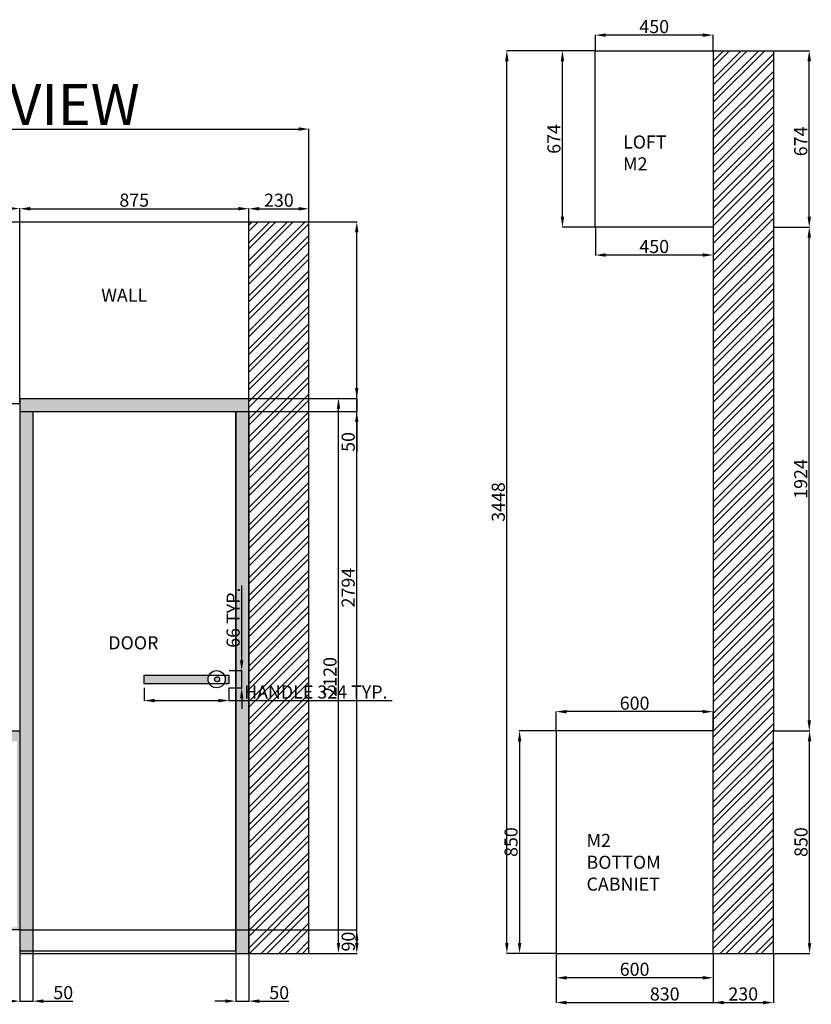
# Model space of a CAD drawing. Units: millimetres. Extents: x 144895 to 155057, y -2833 to 1092.
# Tile 4 of 4: x 152033 to 155057, y -2833 to 929. Entities that reach past the tile are written whole.
import ezdxf

# ---------------------------------------------------------------- set-up
doc = ezdxf.new("R2010")
doc.units = ezdxf.units.MM
for name, color, linetype, lineweight in [('A-ANNO-DIMS', 2, 'Continuous', 18), ('A-ANNO-TEXT', 7, 'Continuous', 18), ('A-DOOR', 4, 'Continuous', 25), ('A-ELEV', 7, 'Continuous', 25), ('A-ELEV-PATT', 252, 'Continuous', 13), ('A-WALL-PATT', 8, 'Continuous', 13)]:
    doc.layers.add(name, color=color, linetype=linetype, lineweight=lineweight)
doc.styles.get("Standard").update_dxf_attribs({"font": 'arial.ttf'})
doc.dimstyles.new('ISO-25', dxfattribs={"dimtxt": 50, "dimasz": 40, "dimexe": 1.25, "dimexo": 0.625, "dimtad": 1, "dimtxsty": 'Standard', "dimcen": 2.5, "dimadec": 0, "dimazin": 0, "dimtfac": 1, "dimtmove": 0, "dimatfit": 3, "dimfxl": 1, "dimarcsym": 0})

# ---------------------------------------------------------------- blocks, each defined once
blk = doc.blocks.new('*D1')
at = {"layer": 'A-ANNO-DIMS', "color": 0, "lineweight": -2, "transparency": 16777216}
for p, q in [((154232, 810.7), (154232, 870.9)), ((154642, 869.6), (154272, 869.6)), ((154682, 810.7), (154682, 870.9))]:
    blk.add_line(p, q, dxfattribs=at)
at = {"layer": 'A-ANNO-DIMS', "color": 0, "transparency": 16777216}
for points in [[(154272, 876.3), (154272, 863), (154232, 869.6)], [(154642, 876.3), (154642, 863), (154682, 869.6)]]:
    blk.add_solid(points, dxfattribs=at)
at = {"layer": 'Defpoints', "color": 0, "transparency": 16777216}
for p in [(154232, 869.6), (154232, 810.1), (154682, 810.1)]:
    blk.add_point(p, dxfattribs=at)
at = {"layer": 'A-ANNO-DIMS', "color": 0, "transparency": 16777216, "insert": (154457, 895.8), "char_height": 50, "attachment_point": 5}
blk.add_mtext('450', dxfattribs=at)
blk = doc.blocks.new('*D2')
at = {"layer": 'A-ANNO-DIMS', "color": 0, "lineweight": -2, "transparency": 16777216}
for p, q in [((154912.6, 810.1), (155050.3, 810.1)), ((155049, 176.1), (155049, 770.1)), ((154912.6, 136.1), (155050.3, 136.1))]:
    blk.add_line(p, q, dxfattribs=at)
at = {"layer": 'A-ANNO-DIMS', "color": 0, "transparency": 16777216}
for points in [[(155042.4, 770.1), (155055.7, 770.1), (155049, 810.1)], [(155042.4, 176.1), (155055.7, 176.1), (155049, 136.1)]]:
    blk.add_solid(points, dxfattribs=at)
at = {"layer": 'Defpoints', "color": 0, "transparency": 16777216}
for p in [(154912, 810.1), (155049, 810.1), (154912, 136.1)]:
    blk.add_point(p, dxfattribs=at)
at = {"layer": 'A-ANNO-DIMS', "color": 0, "transparency": 16777216, "insert": (155022.9, 463.7), "char_height": 50, "attachment_point": 5, "rotation": 90}
blk.add_mtext('674', dxfattribs=at)
blk = doc.blocks.new('*D3')
at = {"layer": 'A-ANNO-DIMS', "color": 0, "lineweight": -2, "transparency": 16777216}
for p, q in [((154082, -2638.5), (154082, -2732.6)), ((154682, -2638.5), (154682, -2732.6)), ((154642, -2731.3), (154122, -2731.3))]:
    blk.add_line(p, q, dxfattribs=at)
at = {"layer": 'A-ANNO-DIMS', "color": 0, "transparency": 16777216}
for points in [[(154122, -2724.7), (154122, -2738), (154082, -2731.3)], [(154642, -2724.7), (154642, -2738), (154682, -2731.3)]]:
    blk.add_solid(points, dxfattribs=at)
at = {"layer": 'Defpoints', "color": 0, "transparency": 16777216}
for p in [(154082, -2637.9), (154682, -2637.9), (154082, -2731.3)]:
    blk.add_point(p, dxfattribs=at)
at = {"layer": 'A-ANNO-DIMS', "color": 0, "transparency": 16777216, "insert": (154382, -2705.2), "char_height": 50, "attachment_point": 5}
blk.add_mtext('600', dxfattribs=at)
blk = doc.blocks.new('*D4')
at = {"layer": 'A-ANNO-DIMS', "color": 0, "lineweight": -2, "transparency": 16777216}
for p, q in [((154912.6, -1787.9), (155051.5, -1787.9)), ((155050.3, -2597.9), (155050.3, -1827.9)), ((154912.6, -2637.9), (155051.5, -2637.9))]:
    blk.add_line(p, q, dxfattribs=at)
at = {"layer": 'A-ANNO-DIMS', "color": 0, "transparency": 16777216}
for points in [[(155043.6, -1827.9), (155057, -1827.9), (155050.3, -1787.9)], [(155043.6, -2597.9), (155057, -2597.9), (155050.3, -2637.9)]]:
    blk.add_solid(points, dxfattribs=at)
at = {"layer": 'Defpoints', "color": 0, "transparency": 16777216}
for p in [(154912, -1787.9), (155050.3, -1787.9), (154912, -2637.9)]:
    blk.add_point(p, dxfattribs=at)
at = {"layer": 'A-ANNO-DIMS', "color": 0, "transparency": 16777216, "insert": (155024.1, -2212.9), "char_height": 50, "attachment_point": 5, "rotation": 90}
blk.add_mtext('850', dxfattribs=at)
blk = doc.blocks.new('*D5')
at = {"layer": 'A-ANNO-DIMS', "color": 0, "lineweight": -2, "transparency": 16777216}
for p, q in [((154081.3, -1787.9), (153941.4, -1787.9)), ((153942.6, -1827.9), (153942.6, -2597.9)), ((154081.3, -2637.9), (153941.4, -2637.9))]:
    blk.add_line(p, q, dxfattribs=at)
at = {"layer": 'A-ANNO-DIMS', "color": 0, "transparency": 16777216}
for points in [[(153935.9, -1827.9), (153949.3, -1827.9), (153942.6, -1787.9)], [(153935.9, -2597.9), (153949.3, -2597.9), (153942.6, -2637.9)]]:
    blk.add_solid(points, dxfattribs=at)
at = {"layer": 'Defpoints', "color": 0, "transparency": 16777216}
for p in [(154082, -1787.9), (153942.6, -2637.9), (154082, -2637.9)]:
    blk.add_point(p, dxfattribs=at)
at = {"layer": 'A-ANNO-DIMS', "color": 0, "transparency": 16777216, "insert": (153916.5, -2212.9), "char_height": 50, "attachment_point": 5, "rotation": 90}
blk.add_mtext('850', dxfattribs=at)
blk = doc.blocks.new('*D6')
at = {"layer": 'A-ANNO-DIMS', "color": 0, "lineweight": -2, "transparency": 16777216}
for p, q in [((154082, -1787.3), (154082, -1713.5)), ((154642, -1714.7), (154122, -1714.7)), ((154682, -1787.3), (154682, -1713.5))]:
    blk.add_line(p, q, dxfattribs=at)
at = {"layer": 'A-ANNO-DIMS', "color": 0, "transparency": 16777216}
for points in [[(154122, -1708.1), (154122, -1721.4), (154082, -1714.7)], [(154642, -1708.1), (154642, -1721.4), (154682, -1714.7)]]:
    blk.add_solid(points, dxfattribs=at)
at = {"layer": 'Defpoints', "color": 0, "transparency": 16777216}
for p in [(154082, -1714.7), (154082, -1787.9), (154682, -1787.9)]:
    blk.add_point(p, dxfattribs=at)
at = {"layer": 'A-ANNO-DIMS', "color": 0, "transparency": 16777216, "insert": (154382, -1688.6), "char_height": 50, "attachment_point": 5}
blk.add_mtext('600', dxfattribs=at)
blk = doc.blocks.new('*D7')
at = {"layer": 'A-ANNO-DIMS', "color": 0, "lineweight": -2, "transparency": 16777216}
for p, q in [((154231.3, 810.1), (154105.2, 810.1)), ((154106.4, 176.1), (154106.4, 770.1)), ((154231.3, 136.1), (154105.2, 136.1))]:
    blk.add_line(p, q, dxfattribs=at)
at = {"layer": 'A-ANNO-DIMS', "color": 0, "transparency": 16777216}
for points in [[(154099.8, 770.1), (154113.1, 770.1), (154106.4, 810.1)], [(154099.8, 176.1), (154113.1, 176.1), (154106.4, 136.1)]]:
    blk.add_solid(points, dxfattribs=at)
at = {"layer": 'Defpoints', "color": 0, "transparency": 16777216}
for p in [(154106.4, 810.1), (154232, 810.1), (154232, 136.1)]:
    blk.add_point(p, dxfattribs=at)
at = {"layer": 'A-ANNO-DIMS', "color": 0, "transparency": 16777216, "insert": (154080.3, 473.1), "char_height": 50, "attachment_point": 5, "rotation": 90}
blk.add_mtext('674', dxfattribs=at)
blk = doc.blocks.new('*D8')
at = {"layer": 'A-ANNO-DIMS', "color": 0, "lineweight": -2, "transparency": 16777216}
for p, q in [((154232, 135.5), (154232, 28.4)), ((154682, 135.5), (154682, 28.4)), ((154642, 29.6), (154272, 29.6))]:
    blk.add_line(p, q, dxfattribs=at)
at = {"layer": 'A-ANNO-DIMS', "color": 0, "transparency": 16777216}
for points in [[(154272, 36.3), (154272, 22.9), (154232, 29.6)], [(154642, 36.3), (154642, 22.9), (154682, 29.6)]]:
    blk.add_solid(points, dxfattribs=at)
at = {"layer": 'Defpoints', "color": 0, "transparency": 16777216}
for p in [(154232, 136.1), (154682, 136.1), (154232, 29.6)]:
    blk.add_point(p, dxfattribs=at)
at = {"layer": 'A-ANNO-DIMS', "color": 0, "transparency": 16777216, "insert": (154457, 55.8), "char_height": 50, "attachment_point": 5}
blk.add_mtext('450', dxfattribs=at)
blk = doc.blocks.new('*D9')
at = {"layer": 'A-ANNO-DIMS', "color": 0, "lineweight": -2, "transparency": 16777216}
for p, q in [((154912.6, 136.1), (155050.3, 136.1)), ((155049, -1747.9), (155049, 96.1)), ((154912.6, -1787.9), (155050.3, -1787.9))]:
    blk.add_line(p, q, dxfattribs=at)
at = {"layer": 'A-ANNO-DIMS', "color": 0, "transparency": 16777216}
for points in [[(155042.4, 96.1), (155055.7, 96.1), (155049, 136.1)], [(155042.4, -1747.9), (155055.7, -1747.9), (155049, -1787.9)]]:
    blk.add_solid(points, dxfattribs=at)
at = {"layer": 'Defpoints', "color": 0, "transparency": 16777216}
for p in [(154912, 136.1), (155049, 136.1), (154912, -1787.9)]:
    blk.add_point(p, dxfattribs=at)
at = {"layer": 'A-ANNO-DIMS', "color": 0, "transparency": 16777216, "insert": (155022.9, -825.9), "char_height": 50, "attachment_point": 5, "rotation": 90}
blk.add_mtext('1924', dxfattribs=at)
blk = doc.blocks.new('*D41')
at = {"layer": 'A-ANNO-DIMS', "color": 0, "lineweight": -2, "ltscale": 20, "transparency": 16777216}
for p, q in [((151570.2, 156.7), (151570.2, 208.4)), ((151993.2, 207.2), (151610.2, 207.2)), ((152033.2, 156.7), (152033.2, 208.4))]:
    blk.add_line(p, q, dxfattribs=at)
at = {"layer": 'A-ANNO-DIMS', "color": 0, "ltscale": 20, "transparency": 16777216}
for points in [[(151610.2, 213.8), (151610.2, 200.5), (151570.2, 207.2)], [(151993.2, 213.8), (151993.2, 200.5), (152033.2, 207.2)]]:
    blk.add_solid(points, dxfattribs=at)
at = {"layer": 'Defpoints', "color": 0, "ltscale": 20, "transparency": 16777216}
for p in [(151570.2, 207.2), (151570.2, 156.1), (152033.2, 156.1)]:
    blk.add_point(p, dxfattribs=at)
at = {"layer": 'A-ANNO-DIMS', "color": 0, "ltscale": 20, "transparency": 16777216, "insert": (151801.7, 233.3), "char_height": 50, "attachment_point": 5}
blk.add_mtext('463', dxfattribs=at)
blk = doc.blocks.new('*D33')
at = {"layer": 'A-ANNO-DIMS', "color": 0, "lineweight": -2, "ltscale": 20, "transparency": 16777216}
for p, q in [((152907.7, -517.9), (153252.2, -517.9)), ((153250.9, -2597.9), (153250.9, -557.9)), ((152908.8, -2637.9), (153252.2, -2637.9))]:
    blk.add_line(p, q, dxfattribs=at)
at = {"layer": 'A-ANNO-DIMS', "color": 0, "ltscale": 20, "transparency": 16777216}
for points in [[(153244.3, -557.9), (153257.6, -557.9), (153250.9, -517.9)], [(153244.3, -2597.9), (153257.6, -2597.9), (153250.9, -2637.9)]]:
    blk.add_solid(points, dxfattribs=at)
at = {"layer": 'Defpoints', "color": 0, "ltscale": 20, "transparency": 16777216}
for p in [(152907, -517.9), (153250.9, -517.9), (152908.2, -2637.9)]:
    blk.add_point(p, dxfattribs=at)
at = {"layer": 'A-ANNO-DIMS', "color": 0, "ltscale": 20, "transparency": 16777216, "insert": (153224.8, -1581.7), "char_height": 50, "attachment_point": 5, "rotation": 90}
blk.add_mtext('2120', dxfattribs=at)
blk = doc.blocks.new('*D38')
at = {"layer": 'A-ANNO-DIMS', "color": 0, "lineweight": -2, "ltscale": 20, "transparency": 16777216}
for p, q in [((152033.2, 156.7), (152033.2, 207.8)), ((152073.2, 206.6), (152868.2, 206.6)), ((152908.2, 156.7), (152908.2, 207.8))]:
    blk.add_line(p, q, dxfattribs=at)
at = {"layer": 'A-ANNO-DIMS', "color": 0, "ltscale": 20, "transparency": 16777216}
for points in [[(152073.2, 213.3), (152073.2, 199.9), (152033.2, 206.6)], [(152868.2, 213.3), (152868.2, 199.9), (152908.2, 206.6)]]:
    blk.add_solid(points, dxfattribs=at)
at = {"layer": 'Defpoints', "color": 0, "ltscale": 20, "transparency": 16777216}
for p in [(152908.2, 206.6), (152033.2, 156.1), (152908.2, 156.1)]:
    blk.add_point(p, dxfattribs=at)
at = {"layer": 'A-ANNO-DIMS', "color": 0, "ltscale": 20, "transparency": 16777216, "insert": (152470.7, 232.8), "char_height": 50, "attachment_point": 5}
blk.add_mtext('875', dxfattribs=at)
blk = doc.blocks.new('*D39')
at = {"layer": 'A-ANNO-DIMS', "color": 0, "lineweight": -2, "ltscale": 20, "transparency": 16777216}
for p, q in [((152908.2, 156.7), (152908.2, 207.6)), ((152948.2, 206.3), (153098.2, 206.3)), ((153138.2, 156.7), (153138.2, 207.6))]:
    blk.add_line(p, q, dxfattribs=at)
at = {"layer": 'A-ANNO-DIMS', "color": 0, "ltscale": 20, "transparency": 16777216}
for points in [[(152948.2, 213), (152948.2, 199.7), (152908.2, 206.3)], [(153098.2, 213), (153098.2, 199.7), (153138.2, 206.3)]]:
    blk.add_solid(points, dxfattribs=at)
at = {"layer": 'Defpoints', "color": 0, "ltscale": 20, "transparency": 16777216}
for p in [(153138.2, 206.3), (152908.2, 156.1), (153138.2, 156.1)]:
    blk.add_point(p, dxfattribs=at)
at = {"layer": 'A-ANNO-DIMS', "color": 0, "ltscale": 20, "transparency": 16777216, "insert": (153023.2, 232.5), "char_height": 50, "attachment_point": 5}
blk.add_mtext('230', dxfattribs=at)
blk = doc.blocks.new('DOOR-HANDLE')
at = {"ltscale": 20}
h = blk.add_hatch(color=256, dxfattribs=at)
h.dxf.hatch_style = 1
h.paths.add_polyline_path([(147980.9, -1557.7), (147732.7, -1557.7), (147732.7, -1591.4), (147982, -1591.4, -0.143725), (147976.8, -1573.6, -0.127114)])
h.paths.add_polyline_path([(148056.8, -1557.7), (148038.3, -1557.7, -0.127123), (148042.5, -1573.6, -0.143716), (148037.2, -1591.4), (148056.8, -1591.4)])
h.paths.add_polyline_path([(148001.6, -1573.7, 1), (148021.1, -1573.7, 1)])
blk.add_lwpolyline([(147732.7, -1557.7), (148056.8, -1557.7), (148056.8, -1591.4), (147732.7, -1591.4)], close=True, dxfattribs=at)
for centre, radius in [((148009.6, -1573.6), 32.8), ((148011.4, -1573.7), 9.79)]:
    blk.add_circle(centre, radius, dxfattribs=at)
blk = doc.blocks.new('*D44')
at = {"layer": 'A-ANNO-DIMS', "color": 0, "lineweight": -2, "ltscale": 20, "transparency": 16777216}
for p, q in [((152508.4, -1624.3), (152508.4, -1673.6)), ((152832.5, -1624.3), (152832.5, -1673.6)), ((152548.4, -1672.3), (152792.5, -1672.3)), ((152832.5, -1672.3), (153456.1, -1672.3))]:
    blk.add_line(p, q, dxfattribs=at)
at = {"layer": 'A-ANNO-DIMS', "color": 0, "ltscale": 20, "transparency": 16777216}
for points in [[(152548.4, -1665.7), (152548.4, -1679), (152508.4, -1672.3)], [(152792.5, -1665.7), (152792.5, -1679), (152832.5, -1672.3)]]:
    blk.add_solid(points, dxfattribs=at)
at = {"layer": 'Defpoints', "color": 0, "ltscale": 20, "transparency": 16777216}
for p in [(152508.4, -1623.7), (152832.5, -1623.7), (152832.5, -1672.3)]:
    blk.add_point(p, dxfattribs=at)
at = {"layer": 'A-ANNO-DIMS', "color": 0, "ltscale": 20, "transparency": 16777216, "insert": (153164.3, -1646.1), "char_height": 50, "attachment_point": 5}
blk.add_mtext('HANDLE 324 TYP.', dxfattribs=at)
blk = doc.blocks.new('*D45')
at = {"layer": 'A-ANNO-DIMS', "color": 0, "lineweight": -2, "ltscale": 20, "transparency": 16777216}
for p, q in [((152881.1, -1518), (152881.1, -1233.1)), ((152833.2, -1558), (152882.4, -1558)), ((152881.1, -1623.7), (152881.1, -1558)), ((152833.2, -1623.7), (152882.4, -1623.7)), ((152881.1, -1663.7), (152881.1, -1703.7))]:
    blk.add_line(p, q, dxfattribs=at)
at = {"layer": 'A-ANNO-DIMS', "color": 0, "ltscale": 20, "transparency": 16777216}
for points in [[(152874.5, -1518), (152887.8, -1518), (152881.1, -1558)], [(152874.5, -1663.7), (152887.8, -1663.7), (152881.1, -1623.7)]]:
    blk.add_solid(points, dxfattribs=at)
at = {"layer": 'Defpoints', "color": 0, "ltscale": 20, "transparency": 16777216}
for p in [(152832.5, -1558), (152881.1, -1558), (152832.5, -1623.7)]:
    blk.add_point(p, dxfattribs=at)
at = {"layer": 'A-ANNO-DIMS', "color": 0, "ltscale": 20, "transparency": 16777216, "insert": (152855, -1355.6), "char_height": 50, "attachment_point": 5, "rotation": 90}
blk.add_mtext('66 TYP.', dxfattribs=at)
blk = doc.blocks.new('*D59')
at = {"layer": 'A-ANNO-DIMS', "color": 0, "lineweight": -2, "ltscale": 20, "transparency": 16777216}
for p, q in [((149913.2, 156.7), (149913.2, 512.1)), ((149953.2, 510.8), (153098.2, 510.8)), ((153138.2, 156.7), (153138.2, 512.1))]:
    blk.add_line(p, q, dxfattribs=at)
at = {"layer": 'A-ANNO-DIMS', "color": 0, "ltscale": 20, "transparency": 16777216}
for points in [[(149953.2, 517.5), (149953.2, 504.2), (149913.2, 510.8)], [(153098.2, 517.5), (153098.2, 504.2), (153138.2, 510.8)]]:
    blk.add_solid(points, dxfattribs=at)
at = {"layer": 'Defpoints', "color": 0, "ltscale": 20, "transparency": 16777216}
for p in [(153138.2, 510.8), (149913.2, 156.1), (153138.2, 156.1)]:
    blk.add_point(p, dxfattribs=at)
at = {"layer": 'A-ANNO-DIMS', "color": 0, "ltscale": 20, "transparency": 16777216, "insert": (151525.7, 537), "char_height": 50, "attachment_point": 5}
blk.add_mtext('3225', dxfattribs=at)
blk = doc.blocks.new('*D60')
at = {"layer": 'A-ANNO-DIMS', "color": 0, "lineweight": -2, "ltscale": 20, "transparency": 16777216}
for p, q in [((153138.8, 156.1), (153321.9, 156.1)), ((153320.7, -2597.9), (153320.7, 116.1)), ((153138.8, -2637.9), (153321.9, -2637.9))]:
    blk.add_line(p, q, dxfattribs=at)
at = {"layer": 'A-ANNO-DIMS', "color": 0, "ltscale": 20, "transparency": 16777216}
for points in [[(153314, 116.1), (153327.4, 116.1), (153320.7, 156.1)], [(153314, -2597.9), (153327.4, -2597.9), (153320.7, -2637.9)]]:
    blk.add_solid(points, dxfattribs=at)
at = {"layer": 'Defpoints', "color": 0, "ltscale": 20, "transparency": 16777216}
for p in [(153138.2, 156.1), (153320.7, 156.1), (153138.2, -2637.9)]:
    blk.add_point(p, dxfattribs=at)
at = {"layer": 'A-ANNO-DIMS', "color": 0, "ltscale": 20, "transparency": 16777216, "insert": (153294.5, -1240.9), "char_height": 50, "attachment_point": 5, "rotation": 90}
blk.add_mtext('2794', dxfattribs=at)
blk = doc.blocks.new('*D62')
at = {"layer": 'A-ANNO-DIMS', "color": 0, "lineweight": -2, "ltscale": 20, "transparency": 16777216}
for p, q in [((151223.2, -2538.5), (151223.2, -2821.7)), ((152033.2, -2638.5), (152033.2, -2821.7)), ((151263.2, -2820.4), (151993.2, -2820.4))]:
    blk.add_line(p, q, dxfattribs=at)
at = {"layer": 'A-ANNO-DIMS', "color": 0, "ltscale": 20, "transparency": 16777216}
for points in [[(151263.2, -2813.8), (151263.2, -2827.1), (151223.2, -2820.4)], [(151993.2, -2813.8), (151993.2, -2827.1), (152033.2, -2820.4)]]:
    blk.add_solid(points, dxfattribs=at)
at = {"layer": 'Defpoints', "color": 0, "ltscale": 20, "transparency": 16777216}
for p in [(151223.2, -2537.9), (152033.2, -2637.9), (152033.2, -2820.4)]:
    blk.add_point(p, dxfattribs=at)
at = {"layer": 'A-ANNO-DIMS', "color": 0, "ltscale": 20, "transparency": 16777216, "insert": (151628.2, -2794.3), "char_height": 50, "attachment_point": 5}
blk.add_mtext('810', dxfattribs=at)
blk = doc.blocks.new('*D67')
at = {"layer": 'A-ANNO-DIMS', "color": 0, "lineweight": -2, "ltscale": 20, "transparency": 16777216}
for p, q in [((152033.8, -2547.9), (153321.9, -2547.9)), ((153320.7, -2587.9), (153320.7, -2597.9)), ((152033.8, -2637.9), (153321.9, -2637.9))]:
    blk.add_line(p, q, dxfattribs=at)
at = {"layer": 'A-ANNO-DIMS', "color": 0, "ltscale": 20, "transparency": 16777216}
for points in [[(153314, -2587.9), (153327.4, -2587.9), (153320.7, -2547.9)], [(153314, -2597.9), (153327.4, -2597.9), (153320.7, -2637.9)]]:
    blk.add_solid(points, dxfattribs=at)
at = {"layer": 'Defpoints', "color": 0, "ltscale": 20, "transparency": 16777216}
for p in [(152033.2, -2547.9), (152033.2, -2637.9), (153320.7, -2637.9)]:
    blk.add_point(p, dxfattribs=at)
at = {"layer": 'A-ANNO-DIMS', "color": 0, "ltscale": 20, "transparency": 16777216, "insert": (153294.5, -2592.9), "char_height": 50, "attachment_point": 5, "rotation": 90}
blk.add_mtext('90', dxfattribs=at)
blk = doc.blocks.new('*D69')
at = {"layer": 'A-ANNO-DIMS', "color": 0, "lineweight": -2, "ltscale": 20, "transparency": 16777216}
for p, q in [((153320.7, -477.9), (153320.7, -437.9)), ((152033.8, -517.9), (153321.9, -517.9)), ((153320.7, -517.9), (153320.7, -567.9)), ((152083.8, -567.9), (153321.9, -567.9)), ((153320.7, -607.9), (153320.7, -720.6))]:
    blk.add_line(p, q, dxfattribs=at)
at = {"layer": 'A-ANNO-DIMS', "color": 0, "ltscale": 20, "transparency": 16777216}
for points in [[(153314, -477.9), (153327.4, -477.9), (153320.7, -517.9)], [(153314, -607.9), (153327.4, -607.9), (153320.7, -567.9)]]:
    blk.add_solid(points, dxfattribs=at)
at = {"layer": 'Defpoints', "color": 0, "ltscale": 20, "transparency": 16777216}
for p in [(152033.2, -517.9), (152083.2, -567.9), (153320.7, -567.9)]:
    blk.add_point(p, dxfattribs=at)
at = {"layer": 'A-ANNO-DIMS', "color": 0, "ltscale": 20, "transparency": 16777216, "insert": (153294.5, -684.3), "char_height": 50, "attachment_point": 5, "rotation": 90}
blk.add_mtext('50', dxfattribs=at)
blk = doc.blocks.new('*D70')
at = {"layer": 'A-ANNO-DIMS', "color": 0, "lineweight": -2, "ltscale": 20, "transparency": 16777216}
for p, q in [((152033.2, -568.5), (152033.2, -2821.7)), ((152083.2, -568.5), (152083.2, -2821.7)), ((151993.2, -2820.4), (151953.2, -2820.4)), ((152033.2, -2820.4), (152083.2, -2820.4)), ((152123.2, -2820.4), (152235.9, -2820.4))]:
    blk.add_line(p, q, dxfattribs=at)
at = {"layer": 'A-ANNO-DIMS', "color": 0, "ltscale": 20, "transparency": 16777216}
for points in [[(151993.2, -2813.8), (151993.2, -2827.1), (152033.2, -2820.4)], [(152123.2, -2813.8), (152123.2, -2827.1), (152083.2, -2820.4)]]:
    blk.add_solid(points, dxfattribs=at)
at = {"layer": 'Defpoints', "color": 0, "ltscale": 20, "transparency": 16777216}
for p in [(152033.2, -567.9), (152083.2, -567.9), (152083.2, -2820.4)]:
    blk.add_point(p, dxfattribs=at)
at = {"layer": 'A-ANNO-DIMS', "color": 0, "ltscale": 20, "transparency": 16777216, "insert": (152199.5, -2794.3), "char_height": 50, "attachment_point": 5}
blk.add_mtext('50', dxfattribs=at)
blk = doc.blocks.new('*D71')
at = {"layer": 'A-ANNO-DIMS', "color": 0, "lineweight": -2, "ltscale": 20, "transparency": 16777216}
for p, q in [((152858.2, -568.5), (152858.2, -2821.7)), ((152908.2, -568.5), (152908.2, -2821.7)), ((152818.2, -2820.4), (152778.2, -2820.4)), ((152858.2, -2820.4), (152908.2, -2820.4)), ((152948.2, -2820.4), (153060.9, -2820.4))]:
    blk.add_line(p, q, dxfattribs=at)
at = {"layer": 'A-ANNO-DIMS', "color": 0, "ltscale": 20, "transparency": 16777216}
for points in [[(152818.2, -2813.8), (152818.2, -2827.1), (152858.2, -2820.4)], [(152948.2, -2813.8), (152948.2, -2827.1), (152908.2, -2820.4)]]:
    blk.add_solid(points, dxfattribs=at)
at = {"layer": 'Defpoints', "color": 0, "ltscale": 20, "transparency": 16777216}
for p in [(152858.2, -567.9), (152908.2, -567.9), (152908.2, -2820.4)]:
    blk.add_point(p, dxfattribs=at)
at = {"layer": 'A-ANNO-DIMS', "color": 0, "ltscale": 20, "transparency": 16777216, "insert": (153024.5, -2794.3), "char_height": 50, "attachment_point": 5}
blk.add_mtext('50', dxfattribs=at)
blk = doc.blocks.new('*D72')
at = {"layer": 'A-ANNO-DIMS', "color": 0, "lineweight": -2, "ltscale": 20, "transparency": 16777216}
for p, q in [((154082, -2638.5), (154082, -2827.2)), ((154912, -2638.5), (154912, -2827.2)), ((154122, -2825.9), (154872, -2825.9))]:
    blk.add_line(p, q, dxfattribs=at)
at = {"layer": 'A-ANNO-DIMS', "color": 0, "ltscale": 20, "transparency": 16777216}
for points in [[(154122, -2819.3), (154122, -2832.6), (154082, -2825.9)], [(154872, -2819.3), (154872, -2832.6), (154912, -2825.9)]]:
    blk.add_solid(points, dxfattribs=at)
at = {"layer": 'Defpoints', "color": 0, "ltscale": 20, "transparency": 16777216}
for p in [(154082, -2637.9), (154912, -2637.9), (154912, -2825.9)]:
    blk.add_point(p, dxfattribs=at)
at = {"layer": 'A-ANNO-DIMS', "color": 0, "ltscale": 20, "transparency": 16777216, "insert": (154497, -2799.7), "char_height": 50, "attachment_point": 5}
blk.add_mtext('830', dxfattribs=at)
blk = doc.blocks.new('*D73')
at = {"layer": 'A-ANNO-DIMS', "color": 0, "lineweight": -2, "ltscale": 20, "transparency": 16777216}
for p, q in [((154231.3, 810.1), (153892.7, 810.1)), ((153894, -2597.9), (153894, 770.1)), ((154081.3, -2637.9), (153892.7, -2637.9))]:
    blk.add_line(p, q, dxfattribs=at)
at = {"layer": 'A-ANNO-DIMS', "color": 0, "ltscale": 20, "transparency": 16777216}
for points in [[(153887.3, 770.1), (153900.6, 770.1), (153894, 810.1)], [(153887.3, -2597.9), (153900.6, -2597.9), (153894, -2637.9)]]:
    blk.add_solid(points, dxfattribs=at)
at = {"layer": 'Defpoints', "color": 0, "ltscale": 20, "transparency": 16777216}
for p in [(153894, 810.1), (154232, 810.1), (154082, -2637.9)]:
    blk.add_point(p, dxfattribs=at)
at = {"layer": 'A-ANNO-DIMS', "color": 0, "ltscale": 20, "transparency": 16777216, "insert": (153867.8, -913.9), "char_height": 50, "attachment_point": 5, "rotation": 90}
blk.add_mtext('3448', dxfattribs=at)
blk = doc.blocks.new('*D74')
at = {"layer": 'A-ANNO-DIMS', "color": 0, "lineweight": -2, "ltscale": 20, "transparency": 16777216}
for p, q in [((154682, -2638.5), (154682, -2827.2)), ((154912, -2638.5), (154912, -2827.2)), ((154722, -2825.9), (154872, -2825.9))]:
    blk.add_line(p, q, dxfattribs=at)
at = {"layer": 'A-ANNO-DIMS', "color": 0, "ltscale": 20, "transparency": 16777216}
for points in [[(154722, -2819.3), (154722, -2832.6), (154682, -2825.9)], [(154872, -2819.3), (154872, -2832.6), (154912, -2825.9)]]:
    blk.add_solid(points, dxfattribs=at)
at = {"layer": 'Defpoints', "color": 0, "ltscale": 20, "transparency": 16777216}
for p in [(154682, -2637.9), (154912, -2637.9), (154912, -2825.9)]:
    blk.add_point(p, dxfattribs=at)
at = {"layer": 'A-ANNO-DIMS', "color": 0, "ltscale": 20, "transparency": 16777216, "insert": (154797, -2799.7), "char_height": 50, "attachment_point": 5}
blk.add_mtext('230', dxfattribs=at)

msp = doc.modelspace()

# ---------------------------------------------------------------- hatches: boundary and pattern name
at = {"layer": 'A-ELEV-PATT', "ltscale": 20}
h = msp.add_hatch(color=256, dxfattribs=at)
h.dxf.hatch_style = 1
h.paths.add_polyline_path([(152083.194, -567.921), (152033.194, -567.921), (152033.194, -2637.921), (152083.194, -2637.921)])
h.paths.add_polyline_path([(152908.194, -517.921), (152033.194, -517.921), (152033.194, -567.921), (152908.194, -567.921)])
h.paths.add_polyline_path([(152908.194, -567.921), (152858.194, -567.921), (152858.194, -2637.921), (152908.194, -2637.921)])
h = msp.add_hatch(color=256, dxfattribs=at)
h.dxf.hatch_style = 1
h.paths.add_polyline_path([(151223.194, -1827.921), (151213.194, -1827.921), (151213.194, -2537.921), (151223.194, -2537.921)], flags=17)
h.paths.add_polyline_path([(151432.009, -1787.921), (150143.194, -1787.921), (150143.194, -2547.921), (152033.194, -2547.921), (152033.194, -1787.921), (151432.009, -1787.921), (151431.804, -1827.921), (151623.194, -1827.921), (152023.194, -1827.921), (152023.194, -2537.921), (151623.194, -2537.921), (151213.194, -2537.921), (150153.194, -2537.921), (150153.194, -1827.921), (151213.194, -1827.921), (151223.194, -1827.921), (151431.804, -1827.921)])
h.paths.add_polyline_path([(150400.933, -2252.777), (150852.877, -2252.777), (150852.877, -2065.556), (150400.933, -2065.556)], flags=25)
at = {"layer": 'A-WALL-PATT'}
h = msp.add_hatch(dxfattribs=at)
h.set_pattern_fill('ANSI32', color=256, scale=5)
h.set_pattern_definition([(45, (-12003.927, -4742.665), (-33.67596, 33.67596), []), (45, (-11981.477, -4742.665), (-33.67596, 33.67596), [])])
h.paths.add_polyline_path([(154911.962, 136.079), (154911.962, 810.079), (154681.962, 810.079), (154681.962, 136.079), (154681.962, -1787.921), (154681.962, -2637.921), (154911.962, -2637.921), (154911.962, -1787.921)])
h = msp.add_hatch(dxfattribs=at)
h.set_pattern_fill('ANSI32', color=256, scale=5)
h.set_pattern_definition([(45, (4775.734, -17.217), (-33.67596, 33.67596), []), (45, (4798.185, -17.217), (-33.67596, 33.67596), [])])
h.paths.add_polyline_path([(152908.194, -2637.921), (153138.194, -2637.921), (153138.194, 156.079), (152908.194, 156.079)])

# ---------------------------------------------------------------- linework, layer by layer
at = {"layer": 'A-ELEV'}
for p, q in [((154231.962, 810.079), (154911.962, 810.079)), ((154231.962, 136.079), (154231.962, 810.079)), ((154681.962, 810.079), (154681.962, 136.079)), ((154911.962, 810.079), (154911.962, 136.079)), ((149913.194, 156.079), (153138.194, 156.079)), ((152033.194, -537.921), (152033.194, 156.079)), ((152908.194, -2637.921), (152908.194, 156.079)), ((153138.194, -2637.921), (153138.194, 156.079)), ((154681.962, 136.079), (154231.962, 136.079)), ((154681.962, 136.079), (154681.962, -1787.921)), ((154911.962, 136.079), (154911.962, -1787.921)), ((152033.194, -517.921), (152033.194, -2637.921)), ((151570.194, -537.921), (152033.194, -537.921)), ((152033.194, -567.921), (152908.194, -567.921)), ((152083.194, -567.921), (152083.194, -2637.921)), ((152858.194, -2627.921), (152858.194, -567.921)), ((150143.194, -1787.921), (152033.194, -1787.921)), ((154681.962, -1787.921), (154081.962, -1787.921)), ((154081.962, -1787.921), (154081.962, -2637.921)), ((154681.962, -2637.921), (154681.962, -1787.921)), ((154911.962, -2637.921), (154911.962, -1787.921)), ((152033.194, -2547.921), (150143.194, -2547.921)), ((152033.194, -2627.921), (152858.194, -2627.921)), ((152033.194, -2637.921), (153138.194, -2637.921)), ((154081.962, -2637.921), (154911.962, -2637.921))]:
    msp.add_line(p, q, dxfattribs=at)

# ---------------------------------------------------------------- block references
at = {"layer": 'A-DOOR'}
msp.add_blockref('DOOR-HANDLE', (4775.734, -17.217), dxfattribs=at)

# ---------------------------------------------------------------- texts
at = {"layer": 'A-ANNO-TEXT', "attachment_point": 1}
for s, width, gutter_width, insert, char_height in [('INNER  VIEW', 9064.84564, 39.102, (151265.645, 682.915), 156.40804), ('LOFT\\PM2', 2897.81963, 12.5, (154337.91, 486.299), 50), ('WALL', 2897.81963, 12.5, (152344.711, -99.039), 50), ('DOOR', 2897.81963, 12.5, (152371.674, -1426.743), 50), ('\\PM2\\PBOTTOM \\PCABNIET', 2897.81963, 12.5, (154198.395, -2098.366), 50)]:
    msp.add_mtext_dynamic_manual_height_columns(s, width=width, gutter_width=gutter_width, heights=[0], dxfattribs=dict(at, insert=insert, char_height=char_height))

# ---------------------------------------------------------------- dimensions: what is measured, and where the dimension line sits
at = {"layer": 'A-ANNO-DIMS'}
dim = msp.add_linear_dim(base=(154231.962, 869.627), p1=(154681.962, 810.079), p2=(154231.962, 810.079), dimstyle='ISO-25', override={"dimclrd": 0, "dimclre": 0, "dimclrt": 0}, dxfattribs=at)
dim.commit()
dim.dimension.update_dxf_attribs({"geometry": '*D1', "text_midpoint": (154456.962, 869.627), "dimtype": 160})
at = {"layer": 'A-ANNO-DIMS', "ltscale": 20}
for base, p1, p2, picture, middle in [((153893.962, 810.079), (154081.962, -2637.921), (154231.962, 810.079), '*D73', (153867.791, -913.921)), ((153320.694, 156.079), (153138.194, -2637.921), (153138.194, 156.079), '*D60', (153294.541, -1240.921)), ((153320.694, -567.921), (152033.194, -517.921), (152083.194, -567.921), '*D69', (153294.541, -684.272)), ((153320.694, -2637.921), (152033.194, -2547.921), (152033.194, -2637.921), '*D67', (153294.541, -2592.921))]:
    dim = msp.add_linear_dim(base=base, p1=p1, p2=p2, angle=90, dimstyle='ISO-25', override={"dimdec": 0, "dimlfac": 1, "dimrnd": 0, "dimzin": 0, "dimdsep": 46, "dimlunit": 2}, dxfattribs=at)
    dim.commit()
    dim.dimension.update_dxf_attribs({"geometry": picture, "text_midpoint": middle})
at = {"layer": 'A-ANNO-DIMS'}
for base, p1, p2, picture, middle in [((154106.421, 810.079), (154231.962, 136.079), (154231.962, 810.079), '*D7', (154080.267, 473.079)), ((155049.035, 136.079), (154911.962, -1787.921), (154911.962, 136.079), '*D9', (155022.881, -825.921)), ((153942.612, -2637.921), (154081.962, -1787.921), (154081.962, -2637.921), '*D5', (153916.459, -2212.921))]:
    dim = msp.add_linear_dim(base=base, p1=p1, p2=p2, angle=90, dimstyle='ISO-25', override={"dimclrd": 0, "dimclre": 0, "dimclrt": 0}, dxfattribs=at)
    dim.commit()
    dim.dimension.update_dxf_attribs({"geometry": picture, "text_midpoint": middle})
for base, p1, p2, picture, middle in [((155049.035, 810.079), (154911.962, 136.079), (154911.962, 810.079), '*D2', (155049.035, 463.702)), ((155050.285, -1787.921), (154911.962, -2637.921), (154911.962, -1787.921), '*D4', (155050.285, -2212.921))]:
    dim = msp.add_linear_dim(base=base, p1=p1, p2=p2, angle=90, dimstyle='ISO-25', override={"dimclrd": 0, "dimclre": 0, "dimclrt": 0}, dxfattribs=at)
    dim.commit()
    dim.dimension.update_dxf_attribs({"geometry": picture, "text_midpoint": middle, "dimtype": 160})
at = {"layer": 'A-ANNO-DIMS', "ltscale": 20}
for base, p1, p2, override, picture, middle in [((153138.194, 510.826), (149913.194, 156.079), (153138.194, 156.079), {"dimdec": 0, "dimlfac": 1, "dimrnd": 0, "dimzin": 0, "dimdsep": 46, "dimlunit": 2}, '*D59', (151525.694, 536.996)), ((151570.194, 207.163), (152033.194, 156.079), (151570.194, 156.079), {"dimclrd": 0, "dimclre": 0, "dimclrt": 0}, '*D41', (151801.694, 233.334)), ((152908.194, 206.597), (152033.194, 156.079), (152908.194, 156.079), {"dimclrd": 0, "dimclre": 0, "dimclrt": 0}, '*D38', (152470.694, 232.75)), ((153138.194, 206.334), (152908.194, 156.079), (153138.194, 156.079), {"dimclrd": 0, "dimclre": 0, "dimclrt": 0}, '*D39', (153023.194, 232.505)), ((152083.194, -2820.421), (152033.194, -567.921), (152083.194, -567.921), {"dimdec": 0, "dimlfac": 1, "dimrnd": 0, "dimzin": 0, "dimdsep": 46, "dimlunit": 2}, '*D70', (152199.546, -2794.267)), ((152908.194, -2820.421), (152858.194, -567.921), (152908.194, -567.921), {"dimdec": 0, "dimlfac": 1, "dimrnd": 0, "dimzin": 0, "dimdsep": 46, "dimlunit": 2}, '*D71', (153024.546, -2794.267)), ((152033.194, -2820.421), (151223.194, -2537.921), (152033.194, -2637.921), {"dimdec": 0, "dimlfac": 1, "dimrnd": 0, "dimzin": 0, "dimdsep": 46, "dimlunit": 2}, '*D62', (151628.194, -2794.267)), ((154911.962, -2825.921), (154081.962, -2637.921), (154911.962, -2637.921), {"dimdec": 0, "dimlfac": 1, "dimrnd": 0, "dimzin": 0, "dimdsep": 46, "dimlunit": 2}, '*D72', (154496.962, -2799.75)), ((154911.962, -2825.921), (154681.962, -2637.921), (154911.962, -2637.921), {"dimdec": 0, "dimlfac": 1, "dimrnd": 0, "dimzin": 0, "dimdsep": 46, "dimlunit": 2}, '*D74', (154796.962, -2799.75))]:
    dim = msp.add_linear_dim(base=base, p1=p1, p2=p2, dimstyle='ISO-25', override=override, dxfattribs=at)
    dim.commit()
    dim.dimension.update_dxf_attribs({"geometry": picture, "text_midpoint": middle})
at = {"layer": 'A-ANNO-DIMS'}
for base, p1, p2, picture, middle in [((154231.962, 29.602), (154681.962, 136.079), (154231.962, 136.079), '*D8', (154456.962, 55.756)), ((154081.962, -1714.741), (154681.962, -1787.921), (154081.962, -1787.921), '*D6', (154381.962, -1688.587)), ((154081.962, -2731.331), (154681.962, -2637.921), (154081.962, -2637.921), '*D3', (154381.962, -2705.177))]:
    dim = msp.add_linear_dim(base=base, p1=p1, p2=p2, dimstyle='ISO-25', override={"dimclrd": 0, "dimclre": 0, "dimclrt": 0}, dxfattribs=at)
    dim.commit()
    dim.dimension.update_dxf_attribs({"geometry": picture, "text_midpoint": middle})
at = {"layer": 'A-ANNO-DIMS', "ltscale": 20}
dim = msp.add_linear_dim(base=(153250.948, -517.921), p1=(152908.194, -2637.921), p2=(152907.032, -517.921), angle=90, dimstyle='ISO-25', override={"dimclrd": 0, "dimclre": 0, "dimclrt": 0}, dxfattribs=at)
dim.commit()
dim.dimension.update_dxf_attribs({"geometry": '*D33', "text_midpoint": (153250.948, -1581.721), "dimtype": 160})
dim = msp.add_linear_dim(base=(152881.148, -1558.013), p1=(152832.535, -1623.705), p2=(152832.535, -1558.013), angle=90, text='<> TYP.', dimstyle='ISO-25', override={"dimdec": 0, "dimrnd": 0, "dimzin": 0, "dimlunit": 2}, dxfattribs=at)
dim.commit()
dim.dimension.update_dxf_attribs({"geometry": '*D45', "text_midpoint": (152854.994, -1355.56)})
dim = msp.add_linear_dim(base=(152832.535, -1672.319), p1=(152508.448, -1623.705), p2=(152832.535, -1623.705), text='HANDLE <> TYP.', dimstyle='ISO-25', override={"dimdec": 0, "dimrnd": 0, "dimzin": 0, "dimlunit": 2}, dxfattribs=at)
dim.commit()
dim.dimension.update_dxf_attribs({"geometry": '*D44', "text_midpoint": (153164.309, -1646.148)})

doc.saveas('drawing.dxf')
